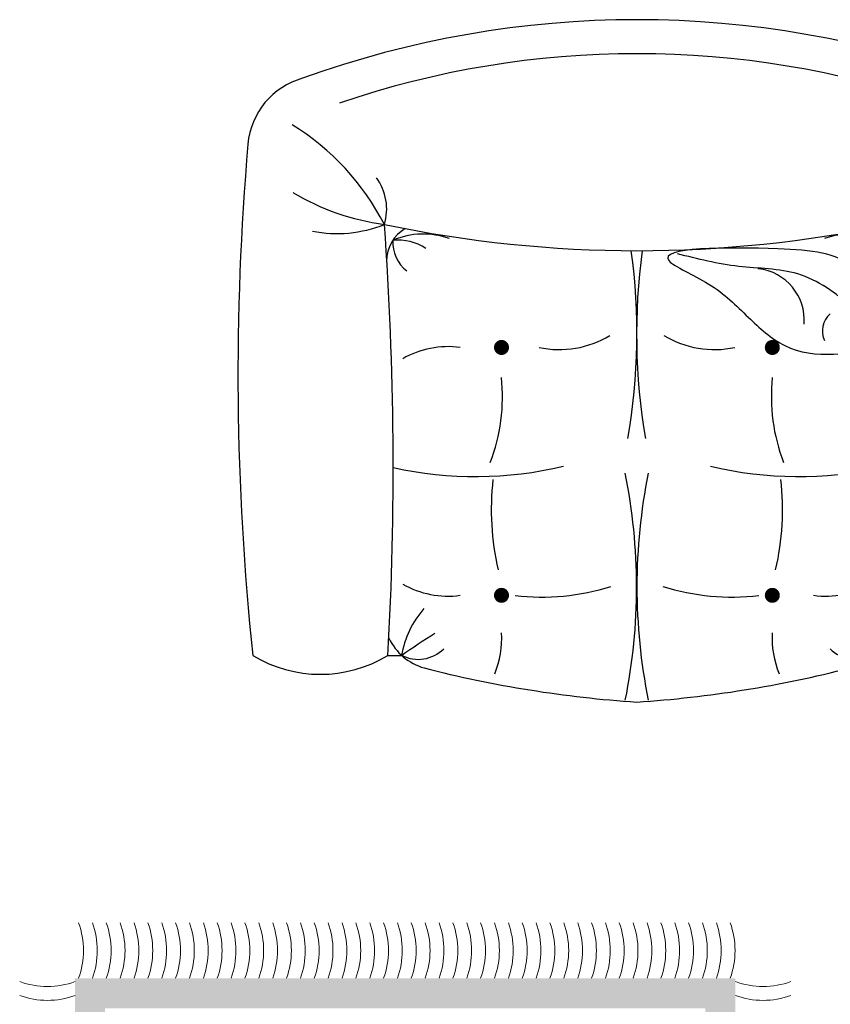
# Model space of a CAD drawing. Units: inches. Extents: x 844 to 2234, y 346 to 1084.
# Tile 41 of 93: x 1249 to 1266, y 708 to 729. Entities that reach past the tile are written whole.
import ezdxf

# ---------------------------------------------------------------- set-up
doc = ezdxf.new("R2010")
doc.units = ezdxf.units.IN
doc.header["$MEASUREMENT"] = 0
doc.layers.add('furniture', color=8, linetype='Continuous', lineweight=18)
doc.layers.add('RA-AP-01$0$INT', color=35, linetype='Continuous', lineweight=5)
doc.layers.add('RA-AP-01$0$FURN', color=3, linetype='Continuous')
doc.layers.add('RA-AP-01$0$WOOD', color=64, linetype='Continuous')

# ---------------------------------------------------------------- blocks, each defined once
blk = doc.blocks.new('A$C18D01794')
at = {"layer": 'RA-AP-01$0$INT'}
h = blk.add_hatch(color=256, dxfattribs=at)
h.paths.add_polyline_path([(4.355206456958071, -6.156712009588037), (4.355206456958071, -8.056712009588038), (5.455206456958072, -8.056712009588038), (5.455206456958072, -6.156712009588037)])
h.paths.add_polyline_path([(4.405206456958072, -8.006712009588039), (4.405206456958072, -6.206712009588038), (5.405206456958072, -6.206712009588038), (5.405206456958072, -8.006712009588039)], flags=16)
for centre, start, end in [((4.309006456945037, -8.156264458284674), 70.20384312815696, 109.7961568705686), ((5.501406456971106, -8.156264458284674), 70.20384312943132, 109.796156871843), ((4.309006456945037, -8.179364458283423), 70.20384312815696, 109.7961568705686), ((5.501406456971106, -8.179364458283423), 70.20384312943132, 109.796156871843), ((4.492158905671144, -8.102912009578965), 160.2038431286875, 199.7961568711004), ((4.515258905666937, -8.102912009582035), 160.2038431286875, 199.7961568711004), ((4.53835890566273, -8.102912009585104), 160.2038431286875, 199.7961568711004), ((4.561458905665799, -8.102912009585218), 160.2038431286875, 199.7961568711004), ((4.584558905661592, -8.102912009588287), 160.2038431286875, 199.7961568711004), ((4.607658905664661, -8.102912009588401), 160.2038431286875, 199.7961568711004), ((4.630758905664774, -8.102912009585673), 160.2038431286875, 199.7961568711004), ((4.653858905660567, -8.102912009588742), 160.2038431286875, 199.7961568711004), ((4.676958905663636, -8.102912009588856), 160.2038431286875, 199.7961568711004), ((4.700058905663976, -8.102912009589083), 160.2038431286875, 199.7961568711004), ((4.723158905662498, -8.102912009586241), 160.2038431286875, 199.7961568711004), ((4.746258905662839, -8.102912009586355), 160.2038431286875, 199.7961568711004), ((4.769358905662952, -8.102912009589536), 160.2038431286875, 199.7961568711004), ((4.792458905660109, -8.102912009586696), 160.2038431286875, 199.7961568711004), ((4.815558905661814, -8.10291200958681), 160.2038431286875, 199.7961568711004), ((4.838658905662154, -8.102912009587037), 160.2038431286875, 199.7961568711004), ((4.861758905665223, -8.102912009590106), 160.2038431286875, 199.7961568711004), ((4.884858905661016, -8.102912009587264), 160.2038431286875, 199.7961568711004), ((4.907958905662721, -8.102912009587492), 160.2038431286875, 199.7961568711004), ((4.931058905658514, -8.102912009590447), 160.2038431286875, 199.7961568711004), ((4.954158905661583, -8.102912009587717), 160.2038431286875, 199.7961568711004), ((4.977258905663288, -8.102912009587946), 160.2038431286875, 199.7961568711004), ((5.000358905663628, -8.102912009587946), 160.2038431286875, 199.7961568711004), ((5.023458905665333, -8.10291200959113), 160.2038431286875, 199.7961568711004), ((5.046558905660899, -8.102912009588287), 160.2038431286875, 199.7961568711004), ((5.069658905661239, -8.102912009588401), 160.2038431286875, 199.7961568711004), ((5.092758905664308, -8.102912009588628), 160.2038431286875, 199.7961568711004), ((5.115858905663057, -8.102912009585786), 160.2038431286875, 199.7961568711004), ((5.13895890566317, -8.102912009588856), 160.2038431286875, 199.7961568711004), ((5.162058905663511, -8.102912009589083), 160.2038431286875, 199.7961568711004), ((5.185158905659076, -8.102912009589197), 160.2038431286875, 199.7961568711004), ((5.208258905660781, -8.102912009586355), 160.2038431286875, 199.7961568711004), ((5.231358905662486, -8.102912009589536), 160.2038431286875, 199.7961568711004), ((5.254458905661235, -8.102912009589652), 160.2038431286875, 199.7961568711004), ((5.277558905661575, -8.102912009589765), 160.2038431286875, 199.7961568711004), ((5.300658905661689, -8.102912009587037), 160.2038431286875, 199.7961568711004), ((5.323758905658846, -8.10291200958715), 160.2038431286875, 199.7961568711004), ((5.346858905659186, -8.10291200959022), 160.2038431286875, 199.7961568711004), ((5.369958905662255, -8.102912009587492), 160.2038431286875, 199.7961568711004), ((5.39305890566396, -8.102912009587492), 160.2038431286875, 199.7961568711004), ((5.416158905664301, -8.102912009587717), 160.2038431286875, 199.7961568711004), ((5.439258905666005, -8.102912009590902), 160.2038431286875, 199.7961568711004), ((5.462358905661571, -8.102912009587946), 160.2038431286875, 199.7961568711004), ((5.485458905657364, -8.10291200958499), 160.2038431286875, 199.7961568711004), ((5.508558905660433, -8.102912009588287), 160.2038431286875, 199.7961568711004), ((5.531658905655999, -8.102912009585332), 160.2038431286875, 199.7961568711004), ((5.554758905651792, -8.102912009582376), 160.2038431286875, 199.7961568711004), ((5.577858905654861, -8.102912009585673), 160.2038431286875, 199.7961568711004)]:
    blk.add_arc(centre, 0.136414042854523, start, end, dxfattribs=at)
blk = doc.blocks.new('A$C7F4351E2')
at = {"layer": 'RA-AP-01$0$FURN'}
for p, q in [((8.352559572600457, -8.263941955512525), (8.35255957259913, -8.282283310927069)), ((8.352559572600457, -8.927748273106442), (8.35255957259913, -8.909406917691898))]:
    blk.add_line(p, q, dxfattribs=at)
at = {"layer": 'RA-AP-01$0$FURN', "const_width": 0.01}
for points in [[(8.437812509519787, -8.415359762755768, 1), (8.427812509519786, -8.415359762755742, 1)], [(8.758197489244363, -8.415359762756214, -1), (8.768197489244365, -8.415359762756214, -1)], [(8.437812509519787, -8.776330465863198, -1), (8.427812509519786, -8.776330465863225, -1)], [(8.758197489244363, -8.776330465862753, 1), (8.768197489244365, -8.776330465862753, 1)]]:
    blk.add_lwpolyline(points, format="xyb", close=True, dxfattribs=at)
at = {"layer": 'RA-AP-01$0$FURN'}
for centre, radius, start, end in [((8.727559572604601, -11.61690445537682), 3.552808610866049, 85.0473312316413, 96.05887237565803), ((8.50205957259015, -8.17394195551301), 0.1744999999876311, 148.9517780040467, 211.048221995953), ((9.025650106946005, -8.176987401637472), 0.1, 15.499494600857, 85.04733123164159), ((8.77247054904813, -7.958543863781743), 0.3382138395168437, 297.2303327094027, 328.2563708342649), ((9.2484631175852, -8.302692737637487), 0.3241573581843151, 149.2985674842688, 172.3026350986055), ((9.084915705374858, -8.196040134964925), 0.1698955038956699, 168.877843135945, 201.8512383801196), ((7.88981694267423, -8.595845114309485), 1.310286319972027, 340.1192502251003, 19.8807497748998), ((7.929864357850293, -8.595845114309483), 1.224941341589781, 341.1257460634955, 18.87425393650447), ((8.947672844970796, -8.191835192646359), 0.0704710051510922, 253.1338634205325, 306.4126496157095), ((8.408522229993444, -8.33300072568355), 0.0753785023123622, 115.8745619060558, 163.9833547230034), ((8.603635103111959, -3.79706073025477), 4.473931917517753, 266.7828902523826, 274.1477233631118), ((8.878389979098333, -8.312202545234353), 0.05, 30.14777190425723, 89.99999999905349), ((10.52713941284929, -8.595845114309466), 1.634931324962266, 168.1200364254424, 191.8799635745573), ((9.101231010340802, -8.38034106221356), 0.5100538472773755, 167.6182489359307, 193.3122231353938), ((8.903279781571525, -8.31837865610295), 0.0478550828899777, 86.575295631534, 142.6833829238214), ((8.838100984994732, -8.276822957859652), 0.0683206773889159, 326.6729861493449, 5.218395042636973), ((8.810121490949696, -8.31110757721543), 0.1042084262671507, 340.4828318717155, 22.86929393278168), ((8.395364730619693, -8.304213854581548), 0.0479292786975047, 152.8070868543555, 225.4025460716553), ((8.333592787569726, -8.402663469525104), 0.1218651776285568, 48.0375529564433, 81.04623209541253), ((7.439612310514541, -8.913795367824825), 1.11020813118073, 31.93286085977143, 34.66647731879807), ((8.553131949433, -8.344109762755968), 0.1214118203512435, 150.1419074485596, 187.691663289156), ((8.642878049331348, -8.344109762756093), 0.1214118203512435, 352.3083367106845, 29.85809255128089), ((9.82633505008426, -8.696671375220811), 1.539060359583382, 165.5338783218257, 176.2437734318419), ((8.374918524725835, -8.294321202996931), 0.1212957045587361, 247.3375839744822, 273.7314750942433), ((8.546954810732721, -8.753394424755975), 0.3517162425384579, 83.41248966761125, 103.1674570565571), ((8.697701155637269, -8.172468128267624), 0.2442261434243043, 248.9017070735605, 275.9923925191661), ((8.73287643248165, -8.469775898206471), 0.3023568492824586, 173.0944825511667, 197.588060785551), ((8.889871101981017, -8.492307869305423), 0.1295083186917369, 167.9901339202812, 211.3796151021958), ((8.444145567704187, -7.829943385268752), 0.765467899454341, 258.6273206109321, 281.4174148186357), ((9.82633505008426, -8.495018853398156), 1.539060359583382, 183.7562265681581, 194.4661216781742), ((8.444145567704187, -9.361312955433425), 0.765467899454341, 78.58258518136427, 101.3726793890678), ((8.781211457338294, -7.772561243483908), 0.8232838708255751, 260.2449188973366, 277.7495311655964), ((8.781211457338294, -9.418695097218269), 0.8232838708255751, 82.25060502413102, 99.75508110266344), ((8.73287643248165, -8.721914330412496), 0.3023568492824586, 162.411939214449, 186.9055174488332), ((8.889871101981017, -8.699382359313544), 0.1295083186917369, 148.6203848978042, 192.0098660797188), ((9.101231010340802, -8.811349166405407), 0.5100538472773755, 166.6877768646062, 192.3817510640693), ((8.799643412436344, -8.749969313933361), 0.0689028341546707, 265.5384273543114, 353.5804828909086), ((8.374918524725835, -8.897369025622035), 0.1212957045587361, 86.26852490575668, 112.6624160255178), ((8.697701155637269, -9.019222100351342), 0.2442261434243043, 84.00760748083387, 111.0982929264395), ((8.546954810732721, -8.438295803862992), 0.3517162425384579, 256.8325429434429, 276.5875103323888), ((8.553131949433, -8.847580465862999), 0.1214118203512435, 172.308336710844, 209.8580925514404), ((8.785133372574222, -8.874256642962408), 0.0310151388417235, 42.62105484496073, 114.2239681486109), ((8.395364730619693, -8.88747637403742), 0.0479292786975047, 134.5974539283447, 207.1929131456445), ((8.810121490949696, -8.880582651403534), 0.1042084262671507, 337.1307060672183, 19.51716812828453), ((7.439612310514541, -8.277894860794142), 1.11020813118073, 325.333522681202, 328.0671391402286), ((8.408522229993444, -8.858689502935416), 0.0753785023123622, 196.0166452769965, 244.1254380939442), ((8.333592787569726, -8.789026759093863), 0.1218651776285568, 278.9537679045875, 311.9624470435567), ((8.838100984994732, -8.914867270759315), 0.0683206773889159, 354.781604957363, 33.32701385065517), ((8.642878049331348, -8.847580465862874), 0.1214118203512435, 330.1419074487191, 340.3913536181062), ((8.903279781571525, -8.873311572516016), 0.0478550828899777, 217.3166170761785, 273.424704368466), ((8.878389979098333, -8.879487683384612), 0.05, 270.0000000009465, 337.4173275753961), ((8.603635103111959, -13.39462949836419), 4.473931917517753, 85.85227663688822, 93.21710974761734), ((8.50205957259015, -9.017748273105955), 0.1744999999876311, 148.9517780040469, 211.0482219959533), ((9.084915705374858, -8.995650093654042), 0.1698955038956699, 158.1487616198804, 191.122156864055), ((8.947672844970796, -8.999855035972608), 0.0704710051510922, 53.58735038429053, 106.8661365794674), ((8.77247054904813, -9.233146364837223), 0.3382138395168437, 31.74362916573515, 62.76966729059727), ((9.2484631175852, -8.88899749098148), 0.3241573581843151, 187.6973649013944, 210.7014325157311), ((9.025650106946005, -9.014702826981493), 0.1, 274.9526687683584, 344.500505399143), ((8.727559572604601, -5.574785773242145), 3.552808610866049, 263.941127624342, 274.9526687683587)]:
    blk.add_arc(centre, radius, start, end, dxfattribs=at)
for points, knots in [([(8.764421239581775, -8.929562504990262), (8.755250524728652, -8.881106864374377), (8.74196437992213, -8.810906376383404), (8.80604948961138, -8.740469753734786), (8.847474678848357, -8.701097198289744), (8.897142214037096, -8.58322730303861), (8.897091569728207, -8.784804210134517), (8.88612504526093, -8.897825917224484), (8.806539053396843, -8.9185794820093), (8.764421239581775, -8.92956250499026)], [0, 0, 0, 0, 0.1367586589314792, 0.1981301758052368, 0.2677729570689282, 0.3281194902553322, 0.4737578340741565, 0.5765194025309516, 0.6920332287422236, 0.6920332287422236, 0.6920332287422236, 0.6920332287422236]), ([(8.764421239581775, -8.92956250499026), (8.782204778269502, -8.914603263160053), (8.821592007255505, -8.881471326160916), (8.86917941606436, -8.814322636989944), (8.867818990542759, -8.729338202119969), (8.881231406199264, -8.676770566934765), (8.888101821971249, -8.649843164808122)], [0, 0, 0, 0, 0.070018540671015, 0.1550780383534498, 0.2344491945777043, 0.3178048737568289, 0.3178048737568289, 0.3178048737568289, 0.3178048737568289])]:
    blk.add_open_spline(points, degree=3, knots=knots, dxfattribs=at)
blk = doc.blocks.new('A$C5D2F253E')
at = {"layer": 'RA-AP-01$0$FURN', "xscale": -0.7999999999883585, "yscale": 0.7999999999883585, "zscale": 0.8, "rotation": 90}
blk.add_blockref('A$C18D01794', (-5.687757199772477, 4.75791982714071), dxfattribs=at)
at = {"layer": 'RA-AP-01$0$WOOD', "xscale": -1, "rotation": 180}
blk.add_blockref('A$C7F4351E2', (-7.164808785335935, -7.45332973198748), dxfattribs=at)

msp = doc.modelspace()

# ---------------------------------------------------------------- block references
at = {"layer": 'furniture', "xscale": -15.94108302203742, "yscale": 15.94108302203742, "zscale": 15.94108302203742, "rotation": 270}
msp.add_blockref('A$C5D2F253E', (1244.08405109492, 696.2584716700112), dxfattribs=at)

doc.saveas('drawing.dxf')
